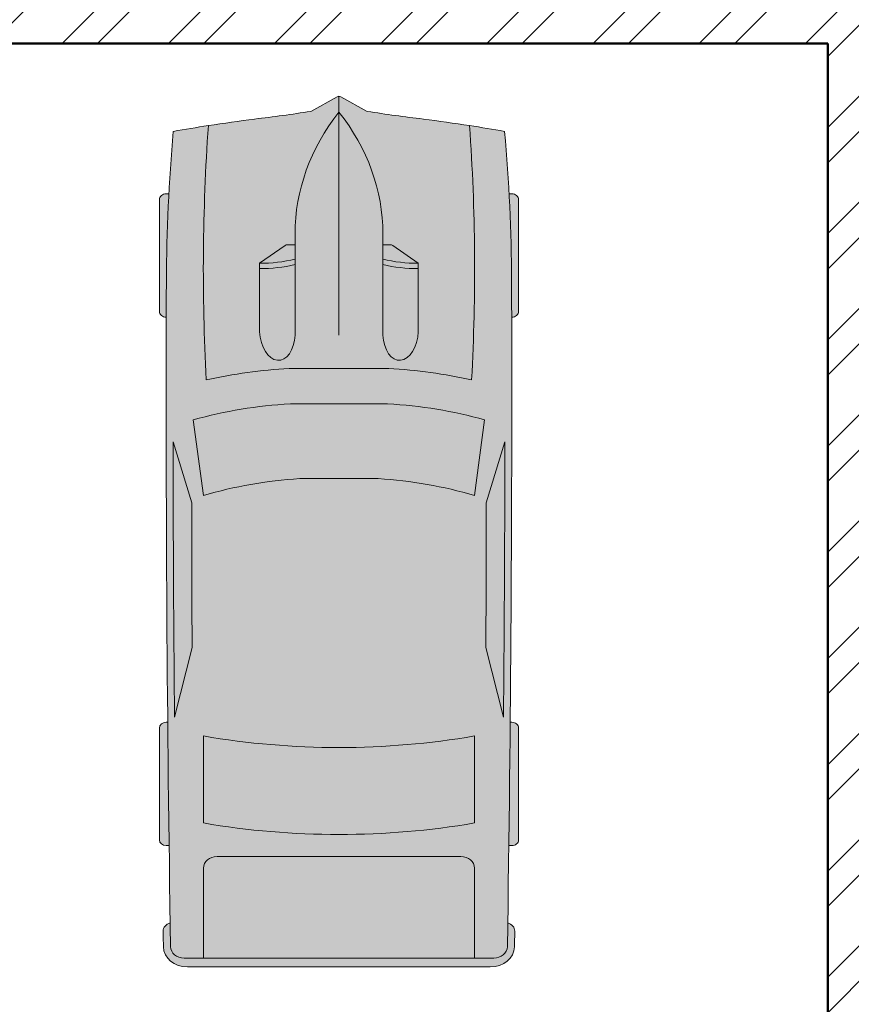
# Model space of a CAD drawing. Units: inches. Extents: x -31485 to -28799, y 18003 to 19130.
# Tile 1 of 15: x -31104 to -30999, y 18273 to 18398. Entities that reach past the tile are written whole.
import ezdxf

# ---------------------------------------------------------------- set-up
doc = ezdxf.new("R2010")
doc.units = ezdxf.units.IN
for name, color, linetype, lineweight in [('A-EQPM', 8, 'Continuous', 18), ('A-WALL', 7, 'Continuous', 50), ('A-WALL-PATT', 8, 'Continuous', 13)]:
    doc.layers.add(name, color=color, linetype=linetype, lineweight=lineweight)

# ---------------------------------------------------------------- blocks, each defined once
blk = doc.blocks.new('*U75')
for p, q in [((1182.463644577746, 987.7673041878503), (567.7039087844591, 987.7673041878503)), ((3472.124202183229, 987.7673041878503), (4086.88393797651, 987.767304187848)), ((536.0433148737552, 950.1792138851854), (536.0433148737552, 935.5404748014407)), ((1214.124238488447, 949.7089586534819), (1214.124238488447, 950.1792138851854)), ((3440.463608272525, 941.6679440245914), (3440.463608272525, 950.1792138851854)), ((4118.544531887212, 950.1792138851804), (4118.544531887212, 934.0601128753084)), ((2234.827175480885, 809.5287016048088), (1898.878785383111, 912.4126225124705)), ((3411.559256322833, 904.3494681924599), (3029.921878250559, 807.1504809911063)), ((4736.411271353851, -850.8646766016326), (4736.411271353883, 850.864676601626)), ((4785.334832293326, -832.0706314503777), (4785.334832293357, 832.0706314502926)), ((1778.76917512805, 801.0177247054045), (2194.716249451875, 745.5217224176465)), ((3515.941238262737, 745.5217224176508), (3994.062813016633, 745.5217224176508)), ((4736.411271353883, 745.5217224176529), (4242.012185201922, 745.5217224176529)), ((4178.690997380514, 670.345541812321), (4178.690997380509, -670.3455418123318)), ((819.5542361210883, 295.2827619512633), (917.6699264680983, 436.1082195367583)), ((917.6699264680983, 436.1082195367583), (1293.848362214069, 436.1082195367583)), ((815.9220749762081, 241.4481679439487), (815.9220749762081, 283.3039660446585)), ((1496.485716216861, -273.6820371142997), (1496.485716216861, 273.6820371142868)), ((756.2288711996046, 241.4481679439487), (1312.764151599097, 241.4481679439487)), ((1690.372337881975, -267.4332505757059), (1690.372337881975, 267.4332505756928)), ((4736.411271353883, -267.4332505757059), (4736.411271353883, 267.4332505756928)), ((2101.521373270556, 215.7994139342878), (2101.521373270556, -215.7994139342835)), ((82.96813941916749, 155.6585683733955), (2.596917328392246, 10.3141998552517)), ((-1.1252e-12, -6.4972e-12), (1312.764151599097, -6.4972e-12)), ((2.596917328392246, -10.31419985525964), (82.96813941916749, -155.6585683734063)), ((756.2288711996046, -241.4481679439617), (1312.764151599097, -241.4481679439617)), ((815.9220749762081, -241.4481679439617), (815.9220749762081, -283.3039660446715)), ((819.5542361210883, -295.2827619512763), (917.6699264680983, -436.1082195367712)), ((917.6699264680983, -436.1082195367712), (1293.848362214069, -436.1082195367712)), ((2194.716249451869, -745.5217224176688), (1778.769175128041, -801.0177247054262)), ((3994.062813016633, -745.5217224176616), (3515.941238262737, -745.5217224176638)), ((4242.012185201917, -745.5217224176638), (4736.411271353857, -745.5217224176594)), ((2234.827175480882, -809.5287016048153), (1898.878785383109, -912.4126225124726)), ((3411.559256322828, -904.349468192473), (3029.921878250557, -807.150480991115)), ((536.0433148737552, -950.1792138851984), (536.0433148737552, -935.5404748014537)), ((1214.124238488447, -949.7089586534948), (1214.124238488447, -950.1792138851984)), ((3440.463608272523, -941.6679440246044), (3440.463608272523, -950.1792138851984)), ((4118.544531887212, -950.1792138851933), (4118.544531887212, -934.0601128753214)), ((1182.463644577746, -987.7673041878633), (567.7039087844591, -987.7673041878633)), ((3472.124202183229, -987.7673041878633), (4086.883937976504, -987.767304187861))]:
    blk.add_line(p, q)
for centre, major_axis, ratio, start_param, end_param in [((567.7039087844591, 950.1792138851861), (5.296e-13, -37.5880903026662), 0.842303869543976, 3.141592653589776, 4.712388980384677), ((1182.463644577746, 950.1792138851861), (5.601e-13, 37.58809030266621), 0.8423038695439758, -1.570796326794884, 1.73e-14), ((3472.124202183229, 950.1792138851861), (5.988e-12, -37.5880903026662), 0.8423038695439762, 3.141592653589603, 4.712388980384554), ((4086.88393797651, 950.179213885181), (1.4197e-12, 37.5880903026662), 0.842303869543976, -1.570796326794865, 4.44e-14), ((1046.255263051279, -12467.92283887244), (3.2861e-12, 13417.14359589015), 0.8423038695439741, 0.0028100083536837, 0.0755983031096952), ((1637.842620806017, -268112.68896731), (4.8454159e-09, 269062.8681811952), 0.842303869543847, -0.0133969486112073, 0.0027970409639888), ((4587.952203166941, 910.2894362332722), (1.8792e-12, 56.38213545399769), 0.8423038695439691, -0.0130174256259048, 1.249894140392862), ((1637.84262086767, -268131.4830124673), (3.42859201765e-05, 269120.9512111412), 0.8423038681351471, -0.0133969484821159, -0.0130174254969711), ((4673.090083532475, 850.8646766015395), (7.5e-15, -75.17618060533067), 0.8423038695439952, 1.570796326796048, 3.128195704978389), ((4673.090083532448, 832.070631450172), (2.1733e-12, -133.2592106239272), 0.8423038695439737, 1.570796326795794, 3.128195704978164), ((6757.162543998887, -699.1204428451242), (4.9938223e-09, 7958.017136535005), 0.8423038695435286, 1.367075990158062, 1.391760499156098), ((1637.842620802809, -268112.6889680619), (4.87113144e-08, -269025.2800916445), 0.8423038695482963, 3.133765086725325, 3.140440689641252), ((3436.395912346701, 136.8410185571553), (5.76965e-11, 2077.023647078763), 0.8423038695439563, 1.245306111696802, 1.507880129813836), ((2433.035484508693, -93125.37499596032), (4.952654e-09, -93935.19844392464), 0.8423038695446962, 3.134048706297306, 3.14409775411291), ((6583.045501169266, -699.1204428451198), (3.826807e-09, -7754.693443154298), 0.8423038695443791, 4.528606069860317, 4.561837674556238), ((951.8333444315502, -15086.63944974413), (1.5767e-12, -15832.53653317094), 0.8423038695439826, 3.09604606856106, 3.200911180495224), ((3413.769624379244, 136.8410185571329), (1.08602e-11, -2280.347340451234), 0.84230386954398, 4.44948196380473, 4.652344057257214), ((3799.722190048092, 71.1058404433382), (2.17448e-11, -2021.323467232052), 0.842303869543983, 4.372215489277867, 4.640744122441986), ((433.884764992104, -3.6096e-12), (1.7438e-12, 3734.255266801694), 0.8423038695439766, 4.511394369635731, 4.913383591133647), ((912.0063397460013, -3.6096e-12), (1.7438e-12, 3734.255266801694), 0.8423038695439766, 4.511394369635731, 4.913383591133647), ((4242.012185201922, 670.3455418123216), (3.5405e-12, 75.17618060533239), 0.842303869543976, 5.55e-14, 1.57079632679492), ((-5194.164488957196, 1330.879982200552), (1.0466145e-09, -6374.389491984369), 0.8423038695441164, 1.385369446298923, 1.434372047871027), ((331.12799165183, 432.0470009052715), (3.125e-11, 696.3661584994836), 0.8423038695439277, 4.435146050259648, 4.718221029521873), ((360.7019022476185, 432.0470009052715), (3.125e-11, 696.3661584994836), 0.8423038695439277, 4.435146050259648, 4.718221029521873), ((1290.073045555822, 338.7781937403542), (161.0379696969085, -9.057857958340485), 0.6038335755719145, -1.39555193967809, 1.581314658479915), ((831.7523719315589, 283.3039660446593), (3.3347e-12, 18.79404515133458), 0.8423038695439091, 0.8797135699495516, 1.570796326795045), ((756.2288711996046, -1185.240851913765), (1.2998e-12, 1426.689019857713), 0.842303869543976, 7e-16, 0.5903187773915901), ((15.83029695535095, -3.6096e-12), (1.9e-15, -18.79404515133476), 0.842303869543842, 4.131459131953847, 5.293318828815531), ((756.2288711996046, 1185.240851913753), (1.01699e-11, 1426.689019857713), 0.8423038695439736, 2.55127387619821, 3.141592653589801), ((-5194.164488957196, -1330.879982200562), (1.0234792e-09, 6374.389491984348), 0.8423038695441192, -1.43437204787103, -1.385369446298926), ((3799.722190048497, -71.10584044329416), (1.038796e-10, -2021.323467232635), 0.8423038695439419, -1.499151468852248, -1.230622835688196), ((331.12799165183, -432.0470009052816), (3.1922e-11, -696.3661584994801), 0.842303869543932, 1.564964277657711, 1.848039256919935), ((360.7019022476185, -432.0470009052816), (3.1922e-11, -696.3661584994801), 0.842303869543932, 1.564964277657711, 1.848039256919935), ((3436.395912346742, -136.8410185572101), (8.13766e-11, -2077.023647078826), 0.8423038695439492, -1.50788012981387, -1.245306111696839), ((831.7523719315589, -283.3039660446737), (3.3028e-12, -18.79404515133458), 0.8423038695439093, 4.712388980384541, 5.403471737230034), ((3413.769624379237, -136.841018557156), (1.090899e-10, -2280.347340451348), 0.8423038695439354, -1.510751403667474, -1.307889310215002), ((6583.045501169163, 699.1204428449458), (2.756795e-10, 7754.693443157768), 0.8423038695439974, 1.721347632622872, 1.754579237318777), ((4242.012185201917, -670.3455418123318), (2.579e-13, -75.17618060533128), 0.8423038695439885, 4.712388980384686, 6.283185307179581), ((6757.162543998887, 699.1204428451076), (2.2231118e-09, 7958.017136528592), 0.8423038695441819, 1.749832154434603, 1.774516663432659), ((951.8333444315729, 15086.63944974408), (2.97009e-11, -15832.5365331709), 0.8423038695439528, -0.0593185269054384, 0.0455465850287298), ((2433.03548450906, 93125.37499596029), (4.1600574e-09, -93935.19844392457), 0.8423038695447548, -0.0025051005232382, 0.007543947292366), ((4673.090083532448, -850.8646766015358), (2.354e-13, 75.17618060532999), 0.8423038695439732, 3.154989602201626, 4.71238898038339), ((4673.090083532349, -832.0706314501077), (6.1679e-12, -133.2592106240062), 0.8423038695439807, 0.0133969486110846, 1.570796326792831), ((1046.255263051284, 12467.92283887242), (3.49903e-10, -13417.14359589015), 0.8423038695440652, -0.0755983031097181, -0.0028100083537155), ((1637.842620803916, 268112.6889680615), (4.0766478e-08, -269025.280091644), 0.8423038695397146, 0.0011519639481523, 0.0078275668641468), ((567.7039087844591, -950.1792138851977), (5.601e-13, 37.58809030266621), 0.8423038695439758, 1.570796326794908, 3.14159265358981), ((1637.842620801787, 268112.6889680619), (1.55395844e-08, 269062.868181947), 0.8423038695458147, 3.138795612625926, 3.154989602201039), ((1182.463644577746, -950.1792138851977), (5.296e-13, -37.5880903026662), 0.842303869543976, -1.69e-14, 1.570796326794884), ((3472.124202183229, -950.1792138851955), (3.96e-13, -37.58809030266733), 0.8423038695440105, -1.570796326794875, -1.27e-14), ((4086.883937976504, -950.1792138851933), (5.0003e-12, 37.58809030266732), 0.8423038695440109, 3.141592653589951, 4.712388980384771), ((4587.952203166856, -910.2894362333229), (5.777e-12, -56.38213545402103), 0.8423038695439803, -1.249894138785958, 0.0130174256254374), ((1637.842620726191, 268131.4830135791), (2.37878358395e-05, 269120.9512123862), 0.8423038705260315, 3.154610079306566, 3.154989602290631)]:
    blk.add_ellipse(centre, major_axis=major_axis, ratio=ratio, start_param=start_param, end_param=end_param)
at = {"extrusion": (0, 0, -1)}
blk.add_ellipse((1290.073045555822, -338.7781937403665), major_axis=(161.0379696969085, 9.057857958340424), ratio=0.6038335755719145, start_param=-1.39555193967809, end_param=1.581314658479915, dxfattribs=at)

msp = doc.modelspace()

# ---------------------------------------------------------------- hatches: boundary and pattern name
at = {"layer": 'A-EQPM'}
h = msp.add_hatch(color=256, dxfattribs=at)
h.dxf.hatch_style = 1
edge = h.paths.add_edge_path()
edge.add_ellipse((-24877.96254945697, 18350.30453975308), major_axis=(6207.481987576119, 3.1368e-12), ratio=0.84230386954367, start_angle=180.3838667787923, end_angle=180.5282714718174, ccw=False)
edge.add_line((-31085.2481756596, 18308.7167228025), (-31085.44453703309, 18308.7167228025))
edge.add_ellipse((-31085.44453703309, 18307.98628917654), major_axis=(-0.8671854094100128, 1.6795e-12), ratio=0.8423038695444475, start_angle=-89.99999999988903, end_angle=1.109639e-10)
edge.add_line((-31086.3117224425, 18307.98628917654), (-31086.3117224425, 18293.8033214099))
edge.add_ellipse((-31085.44453703309, 18293.8033214099), major_axis=(-0.8671854094100128, 3.5068e-12), ratio=0.8423038695402523, start_angle=2.317008e-10, end_angle=90.0000000002317)
edge.add_line((-31085.44453703309, 18293.07288778394), (-31085.07265729416, 18293.07288778394))
edge = h.paths.add_edge_path()
edge.add_ellipse((-31048.05781660086, 18290.22439650316), major_axis=(-1.734370818820025, 1.15572e-11), ratio=0.8423038695444475, start_angle=180.0000000003817, end_angle=270.0000000003818)
edge.add_line((-31048.05781660086, 18291.68526375507), (-31078.9885645288, 18291.68526375507))
edge.add_ellipse((-31078.9885645288, 18290.22439650316), major_axis=(1.734370818820025, 1.15576e-11), ratio=0.8423038695444475, start_angle=89.99999999961817, end_angle=179.9999999996181)
edge.add_line((-31080.72293534762, 18290.22439650316), (-31080.72293534762, 18278.81823911437))
edge.add_line((-31080.72293534762, 18278.81823911437), (-31046.32344578204, 18278.81823911437))
edge.add_line((-31046.32344578204, 18278.81823911437), (-31046.32344578204, 18290.22439650316))
edge = h.paths.add_edge_path()
edge.add_ellipse((-31041.60184409656, 18307.98628917654), major_axis=(0.8671854094100124, 1.6795e-12), ratio=0.8423038695444477, start_angle=-1.109639e-10, end_angle=89.99999999988906)
edge.add_line((-31041.60184409656, 18308.7167228025), (-31041.79820547005, 18308.7167228025))
edge.add_ellipse((-37249.08383165534, 18350.30453975299), major_axis=(6207.481987558772, 4.152598e-10), ratio=0.8423038695472291, start_angle=-0.5282714718218244, end_angle=-0.38386677879640274, ccw=False)
edge.add_line((-31041.97372383549, 18293.07288778394), (-31041.60184409656, 18293.07288778394))
edge.add_ellipse((-31041.60184409656, 18293.8033214099), major_axis=(0.8671854094100124, 3.5068e-12), ratio=0.8423038695402528, start_angle=269.9999999997683, end_angle=359.9999999997682)
edge.add_line((-31040.73465868715, 18293.8033214099), (-31040.73465868715, 18307.98628917654))
edge = h.paths.add_edge_path()
edge.add_ellipse((-31411.5832676395, 18366.13128781071), major_axis=(365.2684817172168, 5.54988e-11), ratio=0.8423038695419378, start_angle=-2.198540565964143, end_angle=2.863714607828726)
edge.add_ellipse((-31079.65242305771, 18236.21500368216), major_axis=(-178.9065886093012, 1.2581094e-09), ratio=0.8423038695391548, start_angle=257.5553727069574, end_angle=259.7904610032577)
edge.add_ellipse((-31032.81879209856, 18507.92406324728), major_axis=(147.0619421407358, 1.9919546e-09), ratio=0.8423038695542743, start_angle=257.4450673550873, end_angle=260.74343399202326, ccw=False)
edge.add_line((-31059.93203075181, 18386.17665916273), (-31063.28523424536, 18388.03088348145))
edge.add_ellipse((-31063.52319056483, 18387.72557949721), major_axis=(-0.4335927046986816, 0), ratio=0.842303869552539, start_angle=232.0668695399768, end_angle=270)
edge.add_line((-31063.52319056483, 18388.09079631018), (-31063.52319056483, 18386.07606494382))
edge.add_ellipse((-31090.86758516267, 18370.64402958174), major_axis=(-32.91478475822442, 2.78257e-11), ratio=0.8423038695443898, start_angle=180.0000000000485, end_angle=209.438569598032, ccw=False)
edge.add_line((-31057.95280040444, 18370.64402958174), (-31057.95280040444, 18369.26686264032))
edge.add_line((-31057.95280040444, 18369.26686264032), (-31056.83106936047, 18369.26686264032))
edge.add_line((-31056.83106936047, 18369.26686264032), (-31053.46184714832, 18366.91946346302))
edge.add_line((-31053.46184714832, 18366.91946346302), (-31053.46184714832, 18358.24074506615))
edge.add_ellipse((-31055.70732377638, 18358.32784445043), major_axis=(0.2089715704820894, 3.715266632531377), ratio=0.6038335755718302, start_angle=106.3425919542722, end_angle=270.9979857249977, ccw=False)
edge.add_line((-31057.95280040444, 18357.80434363074), (-31057.95280040444, 18370.64402958174))
edge.add_ellipse((-31090.86758516267, 18370.64402958174), major_axis=(-32.91478475822442, 2.78257e-11), ratio=0.8423038695443898, start_angle=180.0000000000484, end_angle=209.4385695980319)
edge.add_ellipse((-31036.17879596699, 18370.64402958174), major_axis=(32.91478475822442, 2.78184e-11), ratio=0.8423038695443903, start_angle=150.561430401968, end_angle=179.9999999999515)
edge.add_line((-31069.09358072521, 18370.64402958174), (-31069.09358072521, 18357.80434363074))
edge.add_ellipse((-31071.33905735327, 18358.32784445043), major_axis=(-0.2089715704820894, 3.715266632531377), ratio=0.6038335755718302, start_angle=89.0020142750023, end_angle=253.6574080457279, ccw=False)
edge.add_line((-31073.58453398133, 18358.24074506615), (-31073.58453398133, 18366.91946346302))
edge.add_line((-31073.58453398133, 18366.91946346302), (-31070.21531176918, 18369.26686264032))
edge.add_line((-31070.21531176918, 18369.26686264032), (-31069.09358072521, 18369.26686264032))
edge.add_line((-31069.09358072521, 18369.26686264032), (-31069.09358072521, 18370.64402958174))
edge.add_ellipse((-31036.17879596699, 18370.64402958174), major_axis=(32.91478475822442, 2.78184e-11), ratio=0.8423038695443903, start_angle=150.5614304019681, end_angle=179.9999999999516, ccw=False)
edge.add_line((-31063.52319056483, 18386.07606494382), (-31063.52319056483, 18388.09079631018))
edge.add_ellipse((-31063.52319056483, 18387.72557949721), major_axis=(-0.4335927046986816, 0), ratio=0.842303869552539, start_angle=270, end_angle=307.9331304600232)
edge.add_line((-31063.76114688429, 18388.03088348145), (-31067.11435037783, 18386.17665916273))
edge.add_ellipse((-31094.22758903109, 18507.92406324728), major_axis=(-147.0619421372835, 4.9907306e-09), ratio=0.8423038695736066, start_angle=99.2565660091451, end_angle=102.55493264608151, ccw=False)
edge.add_ellipse((-31047.39395807195, 18236.21500368216), major_axis=(178.9065886092977, 1.2789651e-09), ratio=0.8423038695391513, start_angle=100.209538996733, end_angle=102.4446272930335)
edge.add_ellipse((-30715.46311349015, 18366.13128781071), major_axis=(365.2684817172171, 7.18011e-11), ratio=0.8423038695434502, start_angle=177.1362853921513, end_angle=182.1985405659441)
edge.add_ellipse((-31066.6802154029, 18309.33257301369), major_axis=(52.60932189168197, 7.16232e-11), ratio=0.8423038695431074, start_angle=94.08241069107589, end_angle=107.71995322267611, ccw=False)
edge.add_line((-31069.83724024098, 18353.56574946574), (-31057.20914088867, 18353.56574946574))
edge.add_ellipse((-31060.36616572675, 18309.33257301369), major_axis=(-52.6093218916263, 2.96862e-11), ratio=0.842303869543985, start_angle=252.2800467772827, end_angle=265.9175893088832, ccw=False)
h = msp.add_hatch(color=256, dxfattribs=at)
h.dxf.hatch_style = 1
edge = h.paths.add_edge_path()
edge.add_ellipse((-37249.08383165534, 18350.30453975299), major_axis=(6207.481987558772, 4.152598e-10), ratio=0.8423038695472291, start_angle=-0.3838667787963561, end_angle=0.0902290885904628)
edge.add_ellipse((-37249.08383165534, 18350.30453975299), major_axis=(6207.481987558772, 4.152598e-10), ratio=0.8423038695472291, start_angle=0.0902290885904628, end_angle=0.1349865768543979)
edge.add_ellipse((-31351.16751312684, 18363.95290339437), major_axis=(309.5435567121417, 3.12922e-11), ratio=0.8423038695440732, start_angle=0.1356123904321818, end_angle=2.179950313639523)
edge.add_ellipse((-31351.16751312684, 18363.95290339437), major_axis=(309.5435567121417, 3.12922e-11), ratio=0.8423038695440732, start_angle=2.179950313639523, end_angle=3.650427585692763)
edge.add_ellipse((-31079.65242305771, 18232.19799303183), major_axis=(183.5974185536168, 2.07254122e-08), ratio=0.8423038696260594, start_angle=76.2194710040335, end_angle=77.87403444124779)
edge.add_ellipse((-31411.5832676395, 18366.13128781071), major_axis=(365.2684817172168, 5.54988e-11), ratio=0.8423038695419378, start_angle=-2.1985405659640946, end_angle=2.8637146078286833, ccw=False)
edge.add_ellipse((-31060.36616572675, 18309.33257301369), major_axis=(-52.6093218916263, 2.96862e-11), ratio=0.842303869543985, start_angle=252.2800467772827, end_angle=265.9175893088831)
edge.add_line((-31057.20914088867, 18353.56574946574), (-31069.83724024098, 18353.56574946574))
edge.add_ellipse((-31066.6802154029, 18309.33257301369), major_axis=(52.60932189168197, 7.16232e-11), ratio=0.8423038695431074, start_angle=94.08241069107586, end_angle=107.719953222676)
edge.add_ellipse((-30715.46311349015, 18366.13128781071), major_axis=(365.2684817172171, 7.18011e-11), ratio=0.8423038695434502, start_angle=177.1362853921513, end_angle=182.1985405659441, ccw=False)
edge.add_ellipse((-31047.39395807195, 18232.19799303183), major_axis=(-183.5974185535601, 2.07797544e-08), ratio=0.8423038696263095, start_angle=-77.87403444123211, end_angle=-76.21947100401783)
edge.add_ellipse((-30775.87886800281, 18363.95290339437), major_axis=(-309.5435567121417, 3.20483e-11), ratio=0.8423038695440663, start_angle=-3.650427585692615, end_angle=-2.179950313639383)
edge.add_ellipse((-30775.87886800281, 18363.95290339437), major_axis=(-309.5435567121417, 3.20483e-11), ratio=0.8423038695440663, start_angle=-2.179950313639383, end_angle=-0.1356123904320413)
edge.add_ellipse((-24877.96254945697, 18350.30453975308), major_axis=(6207.481987576119, 3.1368e-12), ratio=0.84230386954367, start_angle=179.8650134231429, end_angle=179.9097709114068)
edge.add_ellipse((-24877.96254945697, 18350.30453975308), major_axis=(6207.481987576119, 3.1368e-12), ratio=0.84230386954367, start_angle=179.9097709114068, end_angle=180.3838667787923)
edge.add_ellipse((-24877.96254945697, 18350.30453975308), major_axis=(6207.481987576119, 3.1368e-12), ratio=0.84230386954367, start_angle=180.3838667787923, end_angle=180.5282714718173)
edge.add_ellipse((-24877.96254945697, 18350.30453975308), major_axis=(6207.481987576119, 3.1368e-12), ratio=0.84230386954367, start_angle=180.5282714718173, end_angle=180.6465540970609)
edge.add_ellipse((-31083.15327623795, 18280.27910636629), major_axis=(1.734370818820398, 6.2835e-12), ratio=0.8423038695442665, start_angle=180.6465540968934, end_angle=269.9999999996497)
edge.add_line((-31083.15327623795, 18278.81823911437), (-31080.72293534762, 18278.81823911437))
edge.add_line((-31080.72293534762, 18278.81823911437), (-31080.72293534762, 18290.41686266714))
edge.add_ellipse((-31078.9885645288, 18290.22439650316), major_axis=(1.734370818820025, 1.15576e-11), ratio=0.8423038695444475, start_angle=89.99999999961818, end_angle=179.9999999996182, ccw=False)
edge.add_line((-31078.9885645288, 18291.68526375507), (-31047.82931692166, 18291.68526375507))
edge.add_ellipse((-31048.05781660086, 18290.22439650316), major_axis=(-1.734370818820025, 1.15572e-11), ratio=0.8423038695444475, start_angle=180.0000000003818, end_angle=270.00000000038176, ccw=False)
edge.add_line((-31046.32344578204, 18290.22439650316), (-31046.32344578204, 18278.81823911437))
edge.add_line((-31046.32344578204, 18278.81823911437), (-31043.8931048917, 18278.81823911437))
edge.add_ellipse((-31043.8931048917, 18280.27910636628), major_axis=(-1.734370818820364, 1.2413e-12), ratio=0.8423038695421853, start_angle=90.00000000018369, end_angle=179.3534459030602)
edge.add_ellipse((-37249.08383165534, 18350.30453975299), major_axis=(6207.481987558772, 4.152598e-10), ratio=0.8423038695472291, start_angle=-0.6465540970657812, end_angle=-0.6186431963230548)
edge.add_ellipse((-37249.08383165534, 18350.30453975299), major_axis=(6207.481987558772, 4.152598e-10), ratio=0.8423038695472291, start_angle=-0.6186431963230548, end_angle=-0.5282714718217923)
edge.add_ellipse((-37249.08383165534, 18350.30453975299), major_axis=(6207.481987558772, 4.152598e-10), ratio=0.8423038695472291, start_angle=-0.5282714718217923, end_angle=-0.3838667787963561)
edge = h.paths.add_edge_path(flags=16)
edge.add_ellipse((-28915.05100716869, 18331.95884452035), major_axis=(2167.155417170915, 1.2045892e-09), ratio=0.8423038695205244, start_angle=179.8791026309351, end_angle=180.3640763488582)
edge.add_line((-31082.14475698858, 18318.18822814799), (-31084.38721045806, 18309.38356786106))
edge.add_ellipse((-24877.96254945698, 18350.30453975303), major_axis=(6206.614802166701, 5.2511138e-09), ratio=0.842303869515611, start_angle=180.0555943134506, end_angle=180.3777641938611, ccw=False)
edge.add_line((-31084.57323347024, 18344.28223983228), (-31082.19962432023, 18336.53165873434))
edge = h.paths.add_edge_path(flags=16)
edge.add_ellipse((-31065.16365558605, 18300.42835811537), major_axis=(46.63344704056234, 1.445442e-10), ratio=0.842303869541784, start_angle=94.8700695969603, end_angle=112.7919148774121)
edge.add_line((-31080.72293534762, 18337.45704785441), (-31082.00326970557, 18347.05325854337))
edge.add_ellipse((-31066.68021540291, 18308.81056759558), major_axis=(47.91849192778146, 1.460375e-10), ratio=0.8423038695419556, start_angle=94.27742096287608, end_angle=111.8349537965307, ccw=False)
edge.add_line((-31069.69307605309, 18349.09263981761), (-31057.35330507656, 18349.09263981761))
edge.add_ellipse((-31060.36616572675, 18308.81056759558), major_axis=(-47.91849192778267, 1.361529e-10), ratio=0.8423038695419347, start_angle=248.1650462034528, end_angle=265.72257903710704, ccw=False)
edge.add_line((-31045.04311142408, 18347.05325854337), (-31046.32344578204, 18337.45704785441))
edge.add_ellipse((-31061.8827255436, 18300.42835811538), major_axis=(-46.63344704055716, 1.546607e-10), ratio=0.8423038695417213, start_angle=247.208085122601, end_angle=265.1299304030565)
edge.add_line((-31058.54453637899, 18339.60712348224), (-31068.50184475066, 18339.60712348224))
edge = h.paths.add_edge_path(flags=16)
edge.add_ellipse((-31063.52319056483, 18378.08074965614), major_axis=(-86.15206721880882, 2.44e-14), ratio=0.8423038695434939, start_angle=76.40186530976904, end_angle=103.5981346902309)
edge.add_line((-31046.32344578204, 18306.97539732048), (-31046.32344578204, 18295.94477431698))
edge.add_ellipse((-31063.52319056483, 18367.05012665263), major_axis=(-86.15206721880666, 5.3e-15), ratio=0.8423038695434728, start_angle=76.40186530976843, end_angle=103.59813469023157, ccw=False)
edge.add_line((-31080.72293534762, 18295.94477431698), (-31080.72293534762, 18306.97539732048))
edge = h.paths.add_edge_path(flags=16)
edge.add_ellipse((-33211.99537396096, 18331.95884452036), major_axis=(-2167.155417170915, 1.2310555e-09), ratio=0.8423038695201377, start_angle=179.6359236511422, end_angle=180.1208973690652)
edge.add_line((-31044.84675680943, 18336.53165873434), (-31042.47314765941, 18344.28223983228))
edge.add_ellipse((-37249.08383167268, 18350.30453975306), major_axis=(-6206.614802166709, 5.3834157e-09), ratio=0.8423038695157945, start_angle=179.6222358061399, end_angle=179.9444056865504, ccw=False)
edge.add_line((-31042.65917067159, 18309.38356786106), (-31044.90162414107, 18318.18822814799))
h = msp.add_hatch(color=256, dxfattribs=at)
h.dxf.hatch_style = 1
edge = h.paths.add_edge_path()
edge.add_ellipse((-31041.60184409656, 18307.98628917654), major_axis=(0.8671854094100124, 1.6795e-12), ratio=0.8423038695444477, start_angle=-1.109639e-10, end_angle=89.99999999988906)
edge.add_line((-31041.60184409656, 18308.7167228025), (-31041.79820547005, 18308.7167228025))
edge.add_ellipse((-37249.08383165534, 18350.30453975299), major_axis=(6207.481987558772, 4.152598e-10), ratio=0.8423038695472291, start_angle=-0.5282714718218244, end_angle=-0.38386677879640274, ccw=False)
edge.add_line((-31041.97372383549, 18293.07288778394), (-31041.60184409656, 18293.07288778394))
edge.add_ellipse((-31041.60184409656, 18293.8033214099), major_axis=(0.8671854094100124, 3.5068e-12), ratio=0.8423038695402528, start_angle=269.9999999997683, end_angle=359.9999999997682)
edge.add_line((-31040.73465868715, 18293.8033214099), (-31040.73465868715, 18307.98628917654))
edge = h.paths.add_edge_path()
edge.add_line((-31085.2481756596, 18308.7167228025), (-31085.44453703309, 18308.7167228025))
edge.add_ellipse((-31085.44453703309, 18307.98628917654), major_axis=(-0.8671854094100128, 1.6795e-12), ratio=0.8423038695444475, start_angle=-89.99999999988903, end_angle=1.109639e-10)
edge.add_line((-31086.3117224425, 18307.98628917654), (-31086.3117224425, 18293.8033214099))
edge.add_ellipse((-31085.44453703309, 18293.8033214099), major_axis=(-0.8671854094100128, 3.5068e-12), ratio=0.8423038695402523, start_angle=2.317008e-10, end_angle=90.0000000002317)
edge.add_line((-31085.44453703309, 18293.07288778394), (-31085.07265729416, 18293.07288778394))
edge.add_ellipse((-24877.96254945697, 18350.30453975308), major_axis=(6207.481987576119, 3.1368e-12), ratio=0.84230386954367, start_angle=180.3838667787923, end_angle=180.5282714718174, ccw=False)
edge = h.paths.add_edge_path()
edge.add_ellipse((-31041.60184409656, 18374.99344173329), major_axis=(0.8671854094100124, 1.6795e-12), ratio=0.8423038695444477, start_angle=-1.109639e-10, end_angle=89.99999999988906)
edge.add_line((-31041.60184409656, 18375.72387535924), (-31041.93957077656, 18375.72387535924))
edge.add_ellipse((-31351.16751312684, 18363.95290339437), major_axis=(309.5435567121417, 3.12922e-11), ratio=0.8423038695440732, start_angle=0.1356123904321862, end_angle=2.1799503136394947, ccw=False)
edge.add_ellipse((-37249.08383165534, 18350.30453975299), major_axis=(6207.481987558772, 4.152598e-10), ratio=0.8423038695472291, start_angle=0.09022908859049039, end_angle=0.13498657685437365, ccw=False)
edge.add_line((-31041.61269323713, 18360.08004034069), (-31041.60184409656, 18360.08004034069))
edge.add_ellipse((-31041.60184409656, 18360.81047396665), major_axis=(-0.8671854094100128, 1.6795e-12), ratio=0.8423038695444475, start_angle=90.00000000011094, end_angle=180.0000000001109)
edge.add_line((-31040.73465868715, 18360.81047396665), (-31040.73465868715, 18374.99344173329))
edge = h.paths.add_edge_path()
edge.add_ellipse((-30775.87886800281, 18363.95290339437), major_axis=(-309.5435567121417, 3.20483e-11), ratio=0.8423038695440663, start_angle=-2.179950313639381, end_angle=-0.13561239043201567, ccw=False)
edge.add_line((-31085.10681035309, 18375.72387535924), (-31085.44453703309, 18375.72387535924))
edge.add_ellipse((-31085.44453703309, 18374.99344173329), major_axis=(-0.8671854094100128, 1.6795e-12), ratio=0.8423038695444475, start_angle=-89.99999999988903, end_angle=1.109639e-10)
edge.add_line((-31086.3117224425, 18374.99344173329), (-31086.3117224425, 18360.81047396665))
edge.add_ellipse((-31085.44453703309, 18360.81047396665), major_axis=(0.8671854094100124, 1.6795e-12), ratio=0.8423038695444477, start_angle=179.999999999889, end_angle=269.999999999889)
edge.add_line((-31085.44453703309, 18360.08004034069), (-31085.43368789252, 18360.08004034069))
edge.add_ellipse((-24877.96254945697, 18350.30453975308), major_axis=(6207.481987576119, 3.1368e-12), ratio=0.84230386954367, start_angle=179.865013423143, end_angle=179.9097709114068, ccw=False)
edge = h.paths.add_edge_path()
edge.add_ellipse((-31053.55554250537, 18379.76913313824), major_axis=(16.06568908904641, 9.1463e-11), ratio=0.8423038695487669, start_angle=251.332504507076, end_angle=270.3967098596572, ccw=False)
edge.add_line((-31057.95280040444, 18366.75368517522), (-31057.95280040444, 18357.80434363074))
edge.add_ellipse((-31055.70732377638, 18358.32784445043), major_axis=(0.2089715704820894, 3.715266632531377), ratio=0.6038335755718302, start_angle=106.3425919542721, end_angle=270.9979857249977)
edge.add_line((-31053.46184714832, 18358.24074506615), (-31053.46184714832, 18366.23717118477))
edge = h.paths.add_edge_path()
edge.add_ellipse((-31056.98715577818, 18368.90164582734), major_axis=(-0.4335927047225754, 4.1219e-11), ratio=0.8423038695061223, start_angle=225.5197891228621, end_angle=270.0000000054467)
edge.add_line((-31056.98715577818, 18369.26686264032), (-31057.95280040444, 18369.26686264032))
edge.add_line((-31057.95280040444, 18369.26686264032), (-31057.95280040444, 18367.43597745348))
edge.add_ellipse((-31053.55554250537, 18380.4514254165), major_axis=(-16.06568908915088, 3.60949e-11), ratio=0.8423038695435023, start_angle=71.33250450753091, end_angle=90.39670986011207)
edge.add_line((-31053.46184714832, 18366.91946346302), (-31056.71079598047, 18369.183065961))
edge = h.paths.add_edge_path()
edge.add_line((-31069.09358072521, 18369.26686264032), (-31070.05922535147, 18369.26686264032))
edge.add_ellipse((-31070.05922535147, 18368.90164582734), major_axis=(0.4335927047225755, 4.12191e-11), ratio=0.8423038695061222, start_angle=89.99999999455322, end_angle=134.4802108771379)
edge.add_line((-31070.33558514919, 18369.183065961), (-31073.58453398133, 18366.91946346302))
edge.add_ellipse((-31073.49083862428, 18380.4514254165), major_axis=(16.06568908915091, 3.60949e-11), ratio=0.8423038695435009, start_angle=269.6032901398879, end_angle=288.6674954924691)
edge.add_line((-31069.09358072521, 18367.43597745348), (-31069.09358072521, 18369.26686264032))
edge = h.paths.add_edge_path()
edge.add_ellipse((-31073.49083862428, 18379.76913313824), major_axis=(-16.06568908904639, 9.1463e-11), ratio=0.8423038695487673, start_angle=89.60329014034278, end_angle=108.66749549292399, ccw=False)
edge.add_line((-31073.58453398133, 18366.23717118477), (-31073.58453398133, 18358.24074506615))
edge.add_ellipse((-31071.33905735327, 18358.32784445043), major_axis=(-0.2089715704820894, 3.715266632531377), ratio=0.6038335755718302, start_angle=89.00201427500228, end_angle=253.6574080457278)
edge.add_line((-31069.09358072521, 18357.80434363074), (-31069.09358072521, 18366.75368517522))
h = msp.add_hatch(color=256, dxfattribs=at)
h.dxf.hatch_style = 1
edge = h.paths.add_edge_path()
edge.add_ellipse((-31053.55554250537, 18380.4514254165), major_axis=(-16.06568908915088, 3.60949e-11), ratio=0.8423038695435023, start_angle=71.33250450753093, end_angle=90.39670986011208, ccw=False)
edge.add_line((-31057.95280040444, 18367.43597745348), (-31057.95280040444, 18366.75368517522))
edge.add_ellipse((-31053.55554250537, 18379.76913313824), major_axis=(16.06568908904641, 9.1463e-11), ratio=0.8423038695487669, start_angle=251.332504507076, end_angle=270.3967098596572)
edge.add_line((-31053.46184714832, 18366.23717118477), (-31053.46184714832, 18366.91946346302))
edge = h.paths.add_edge_path()
edge.add_ellipse((-31073.49083862428, 18380.4514254165), major_axis=(16.06568908915091, 3.60949e-11), ratio=0.8423038695435009, start_angle=269.6032901398879, end_angle=288.667495492469, ccw=False)
edge.add_line((-31073.58453398133, 18366.91946346302), (-31073.58453398133, 18366.23717118477))
edge.add_ellipse((-31073.49083862428, 18379.76913313824), major_axis=(-16.06568908904639, 9.1463e-11), ratio=0.8423038695487673, start_angle=89.60329014034272, end_angle=108.667495492924)
edge.add_line((-31069.09358072521, 18366.75368517522), (-31069.09358072521, 18367.43597745348))
h = msp.add_hatch(color=256, dxfattribs=at)
h.dxf.hatch_style = 1
edge = h.paths.add_edge_path()
edge.add_ellipse((-31060.36616572675, 18308.81056759558), major_axis=(-47.91849192778267, 1.361529e-10), ratio=0.8423038695419347, start_angle=248.1650462034528, end_angle=265.722579037107)
edge.add_line((-31057.35330507656, 18349.09263981761), (-31069.69307605309, 18349.09263981761))
edge.add_ellipse((-31066.68021540291, 18308.81056759558), major_axis=(47.91849192778146, 1.460375e-10), ratio=0.8423038695419556, start_angle=94.277420962876, end_angle=111.8349537965306)
edge.add_line((-31082.00326970557, 18347.05325854337), (-31080.72293534762, 18337.45704785441))
edge.add_ellipse((-31065.16365558605, 18300.42835811537), major_axis=(46.63344704056234, 1.445442e-10), ratio=0.842303869541784, start_angle=94.8700695969602, end_angle=112.7919148774121, ccw=False)
edge.add_line((-31068.50184475066, 18339.60712348224), (-31058.54453637899, 18339.60712348224))
edge.add_ellipse((-31061.8827255436, 18300.42835811538), major_axis=(-46.63344704055716, 1.546607e-10), ratio=0.8423038695417213, start_angle=247.20808512260112, end_angle=265.1299304030565, ccw=False)
edge.add_line((-31046.32344578204, 18337.45704785441), (-31045.04311142408, 18347.05325854337))
edge = h.paths.add_edge_path()
edge.add_ellipse((-28915.05100716869, 18331.95884452035), major_axis=(2167.155417170915, 1.2045892e-09), ratio=0.8423038695205244, start_angle=179.8791026309352, end_angle=180.3640763488582, ccw=False)
edge.add_line((-31082.19962432023, 18336.53165873434), (-31084.57323347024, 18344.28223983228))
edge.add_ellipse((-24877.96254945698, 18350.30453975303), major_axis=(6206.614802166701, 5.2511138e-09), ratio=0.842303869515611, start_angle=180.0555943134505, end_angle=180.377764193861)
edge.add_line((-31084.38721045806, 18309.38356786106), (-31082.14475698858, 18318.18822814799))
edge = h.paths.add_edge_path()
edge.add_ellipse((-37249.08383167268, 18350.30453975306), major_axis=(-6206.614802166709, 5.3834157e-09), ratio=0.8423038695157945, start_angle=179.6222358061398, end_angle=179.9444056865503)
edge.add_line((-31042.47314765941, 18344.28223983228), (-31044.84675680943, 18336.53165873434))
edge.add_ellipse((-33211.99537396096, 18331.95884452036), major_axis=(-2167.155417170915, 1.2310555e-09), ratio=0.8423038695201377, start_angle=179.6359236511423, end_angle=180.1208973690653, ccw=False)
edge.add_line((-31044.90162414107, 18318.18822814799), (-31042.65917067159, 18309.38356786106))
edge = h.paths.add_edge_path()
edge.add_ellipse((-31063.52319056483, 18378.08074965614), major_axis=(-86.15206721880882, 2.44e-14), ratio=0.8423038695434939, start_angle=76.40186530976911, end_angle=103.598134690231, ccw=False)
edge.add_line((-31080.72293534762, 18306.97539732048), (-31080.72293534762, 18295.94477431698))
edge.add_ellipse((-31063.52319056483, 18367.05012665263), major_axis=(-86.15206721880666, 5.3e-15), ratio=0.8423038695434728, start_angle=76.40186530976838, end_angle=103.5981346902316)
edge.add_line((-31046.32344578204, 18295.94477431698), (-31046.32344578204, 18306.97539732048))
edge = h.paths.add_edge_path()
edge.add_ellipse((-31044.3266975964, 18280.27910636629), major_axis=(3.074389845080431, 4.5193e-12), ratio=0.8423038695441155, start_angle=269.9999999999962, end_angle=359.3534459027799)
edge.add_ellipse((-37249.51742436018, 18350.30453975157), major_axis=(6208.82200659716, 5.2733622375e-06), ratio=0.8423038788855755, start_angle=-0.646554145712032, end_angle=-0.6282372648788858)
edge.add_ellipse((-31042.52213115786, 18282.24330106324), major_axis=(-1.30077811411332, 2.65586e-11), ratio=0.8423038695457158, start_angle=179.3717627849924, end_angle=248.4647566023133)
edge.add_ellipse((-37249.08383165534, 18350.30453975299), major_axis=(6207.481987558772, 4.152598e-10), ratio=0.8423038695472291, start_angle=-0.6465540970658026, end_angle=-0.6186431963230916, ccw=False)
edge.add_ellipse((-31043.8931048917, 18280.27910636628), major_axis=(-1.734370818820364, 1.2413e-12), ratio=0.8423038695421853, start_angle=90.00000000018372, end_angle=179.3534459030602, ccw=False)
edge.add_line((-31043.8931048917, 18278.81823911437), (-31083.15327623795, 18278.81823911437))
edge.add_ellipse((-31083.15327623795, 18280.27910636629), major_axis=(1.734370818820398, 6.2835e-12), ratio=0.8423038695442665, start_angle=180.6465540968934, end_angle=269.99999999964973, ccw=False)
edge.add_ellipse((-24877.96254945697, 18350.30453975308), major_axis=(6207.481987576119, 3.1368e-12), ratio=0.84230386954367, start_angle=180.5282714718174, end_angle=180.6465540970609, ccw=False)
edge.add_ellipse((-31084.5242499718, 18282.24330106324), major_axis=(1.300778114113422, 3.7711e-12), ratio=0.8423038695465029, start_angle=111.5352435038071, end_angle=180.6282372160113)
edge.add_ellipse((-24877.52895674383, 18350.30453975483), major_axis=(-6208.822006624284, 5.909233014e-06), ratio=0.842303880027109, start_angle=0.6282372707742053, end_angle=0.6465541516072572)
edge.add_ellipse((-31082.71968353324, 18280.27910636629), major_axis=(-3.074389845084005, 2.9376e-12), ratio=0.8423038695431365, start_angle=0.6465540971220629, end_angle=89.99999999989375)
edge.add_line((-31082.71968353325, 18277.68953590329), (-31044.3266975964, 18277.68953590329))
at = {"layer": 'A-WALL-PATT'}
h = msp.add_hatch(dxfattribs=at)
h.set_pattern_fill('ANSI32', color=256)
h.set_pattern_definition([(45, (-1687.357050595019, -0.3129728357926069), (-6.735192090801865, 6.735192090801866), []), (45, (-1682.866920595021, -0.3129728357926069), (-6.735192090801865, 6.735192090801866), [])])
h.paths.add_polyline_path([(-31156.52828769349, 18823.80296009311), (-31209.52828769349, 18823.80296009311), (-31209.52828769349, 18761.80296009311), (-31200.52828769349, 18761.80296009311), (-31200.52828769349, 18814.80296009311), (-31156.52828769349, 18814.80296009311)], flags=17)
h.paths.add_polyline_path([(-31022.5282876935, 18823.80296009311), (-31118.52828769349, 18823.80296009311), (-31118.52828769349, 18814.80296009311), (-31074.52828769349, 18814.80296009311), (-31074.52828769349, 18720.78574754094), (-31070.95696393926, 18720.78574754094), (-31068.52828769349, 18720.75952290947), (-31068.52828769349, 18814.80296009311), (-31022.5282876935, 18814.80296009311)], flags=17)
h.paths.add_polyline_path([(-30754.52828769349, 18823.80296009311), (-30850.5282876935, 18823.80296009311), (-30850.5282876935, 18814.80296009311), (-30806.5282876935, 18814.80296009311), (-30806.52828769349, 18723.10029278397), (-30800.5282876935, 18723.10029278397), (-30800.5282876935, 18814.80296009311), (-30754.52828769349, 18814.80296009311)], flags=17)
h.paths.add_polyline_path([(-30661.52828769349, 18823.80296009311), (-30716.52828769349, 18823.80296009311), (-30716.52828769349, 18814.80296009311), (-30670.52828769349, 18814.80296009311), (-30670.52828769349, 18761.80296009311), (-30661.52828769349, 18761.80296009311)], flags=17)
h.paths.add_polyline_path([(-30986.91891278487, 18670.80296009311), (-31068.52828769349, 18670.80296009311), (-31068.52828769349, 18684.75952290947), (-31074.52828769349, 18684.75952290947), (-31074.52828769349, 18670.80296009311), (-31200.52828769349, 18670.80296009311), (-31200.52828769349, 18723.80296009311), (-31209.52828769349, 18723.80296009311), (-31209.52828769349, 18641.80296009311), (-31200.52828769349, 18641.80296009311), (-31200.52828769349, 18664.80296009311), (-31104.52828769349, 18664.80296009311), (-31104.52828769349, 18628.92834044014), (-31098.52828769349, 18628.92834044014), (-31098.52828769348, 18664.8029600931), (-30986.91891278488, 18664.8029600931)], flags=17)
h.paths.add_polyline_path([(-30661.52828769349, 18723.80296009311), (-30670.52828769349, 18723.80296009311), (-30670.52828769349, 18670.80296009311), (-30800.5282876935, 18670.80296009311), (-30800.5282876935, 18687.10029278396), (-30806.52828769349, 18687.10029278396), (-30806.52828769349, 18670.80296009311), (-30885.59628027248, 18670.80296009311), (-30885.59628027248, 18667.80293426455), (-30885.59628027248, 18664.80296009311), (-30760.52828769349, 18664.80296009311), (-30760.52828769349, 18625.80296009311), (-30754.52828769349, 18625.80296009311), (-30754.52828769349, 18664.80296009311), (-30670.52828769349, 18664.80296009311), (-30670.52828769349, 18641.80296009311), (-30661.52828769349, 18641.80296009311)], flags=17)
h.paths.add_polyline_path([(-31200.52828769349, 18574.80296009311), (-31188.56436894977, 18574.80296009311), (-31188.56436894977, 18580.80296009311), (-31200.52828769349, 18580.80296009311), (-31200.52828769349, 18603.80296009311), (-31209.52828769349, 18603.80296009311), (-31209.52828769349, 18557.80296009311), (-31200.52828769349, 18557.80296009311)], flags=17)
h.paths.add_polyline_path([(-31098.52828769349, 18592.92834044014), (-31104.52828769349, 18592.92834044014), (-31104.52828769349, 18580.80296009311), (-31164.56436894977, 18580.80296009311), (-31164.56436894977, 18574.80296009311), (-31104.52828769349, 18574.80296009311), (-31104.52828769349, 18514.80296009311), (-31200.52828769349, 18514.80296009311), (-31200.52828769349, 18531.80296009311), (-31209.52828769349, 18531.80296009311), (-31209.52828769349, 18473.80296009311), (-31200.52828769349, 18473.80296009311), (-31200.52828769349, 18508.80296009311), (-31056.52828769349, 18508.80296009312), (-31056.52828769349, 18501.62307445529), (-31050.52828769349, 18501.62307445529), (-31050.52828769349, 18514.80296009311), (-31098.52828769349, 18514.80296009311)], flags=17)
h.paths.add_polyline_path([(-30661.52828769349, 18531.80296009311), (-30670.52828769349, 18531.80296009311), (-30670.52828769349, 18514.80296009311), (-30754.52828769349, 18514.80296009311), (-30754.52828769349, 18574.80296009311), (-30700.74522746605, 18574.80296009311), (-30700.74522746605, 18577.44024221289), (-30700.74522746605, 18580.8029600931), (-30754.52828769349, 18580.80296009311), (-30754.52828769349, 18589.80296009311), (-30760.52828769349, 18589.80296009311), (-30760.52828769349, 18514.80296009311), (-30820.52828769349, 18514.80296009311), (-30820.52828769348, 18499.26438911774), (-30814.52828769349, 18499.26438911774), (-30814.52828769349, 18508.80296009311), (-30670.52828769349, 18508.80296009311), (-30670.52828769349, 18473.80296009311), (-30661.52828769349, 18473.80296009311)], flags=17)
h.paths.add_polyline_path([(-30661.52828769349, 18435.80296009311), (-30670.52828769349, 18435.80296009311), (-30670.52828769349, 18400.80296009311), (-30814.52828769349, 18400.80296009311), (-30814.52828769349, 18413.15176302367), (-30820.52828769349, 18413.15176302367), (-30820.52828769349, 18400.80296009311), (-30932.52828769349, 18400.80296009311), (-30932.52828769349, 18664.80296009311), (-30921.59628027248, 18664.80296009311), (-30921.59628027248, 18670.80296009311), (-30932.5282876935, 18670.80296009311), (-30932.5282876935, 18814.80296009311), (-30888.5282876935, 18814.80296009311), (-30888.5282876935, 18823.80296009311), (-30984.5282876935, 18823.80296009311), (-30984.5282876935, 18814.80296009311), (-30938.5282876935, 18814.80296009311), (-30938.5282876935, 18670.80296009311), (-30950.91891278487, 18670.80296009311), (-30950.91891278488, 18664.80296009311), (-30938.5282876935, 18664.80296009311), (-30938.52828769349, 18400.80296009311), (-31050.52828769349, 18400.80296009311), (-31050.52828769349, 18411.18080736427), (-31056.52828769348, 18411.18080736427), (-31056.52828769348, 18400.80296009311), (-31200.52828769349, 18400.80296009311), (-31200.52828769349, 18435.80296009311), (-31209.52828769349, 18435.80296009311), (-31209.52828769349, 18179.80296009311), (-31200.52828769349, 18179.80296009311), (-31200.52828769349, 18394.80296009311), (-31001.52828769348, 18394.80296009311), (-31001.52828769348, 18179.80296009311), (-30954.52828769347, 18179.80296009311), (-30954.52828769347, 18188.80296009311), (-30995.52828769348, 18188.80296009311), (-30995.52828769348, 18394.80296009311), (-30875.52828769348, 18394.80296009311), (-30875.52828769348, 18188.80296009311), (-30916.52828769347, 18188.80296009311), (-30916.52828769347, 18179.80296009311), (-30869.52828769348, 18179.80296009311), (-30869.52828769348, 18394.80296009311), (-30670.52828769349, 18394.80296009311), (-30670.52828769349, 18179.80296009311), (-30661.52828769349, 18179.80296009311)])

# ---------------------------------------------------------------- linework, layer by layer
at = {"layer": 'A-WALL'}
for p, q in [((-31200.52828769349, 18394.80296009311), (-31001.52828769348, 18394.80296009311)), ((-31001.52828769348, 18394.80296009311), (-31001.52828769348, 18179.80296009311))]:
    msp.add_line(p, q, dxfattribs=at)

# ---------------------------------------------------------------- block references
at = {"layer": 'A-EQPM', "xscale": 0.0230707493364654, "yscale": 0.0230707493364654, "zscale": 0.0230707493364654, "rotation": 270}
msp.add_blockref('*U75', (-31063.52319056483, 18388.09079631018), dxfattribs=at)

doc.saveas('drawing.dxf')
